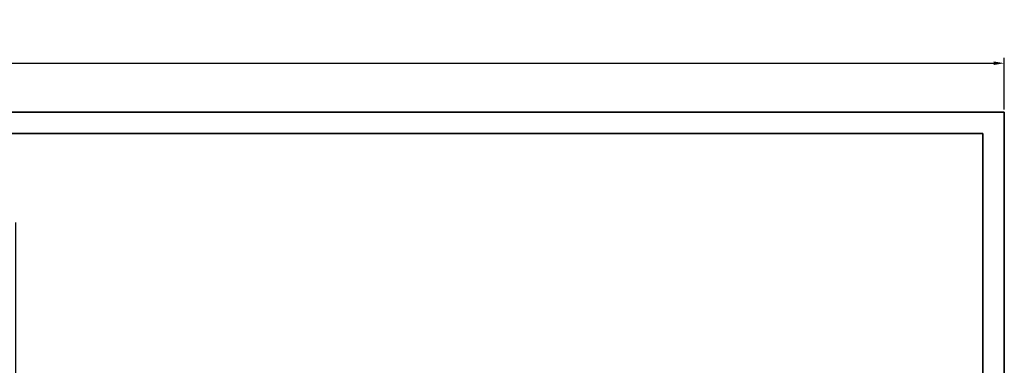
# Model space of a CAD drawing. Units: inches. Extents: x 3008 to 4088, y 1255 to 2137.
# Tile 30 of 30: x 3853 to 4083, y 1951 to 2031. Entities that reach past the tile are written whole.
import ezdxf

# ---------------------------------------------------------------- set-up
doc = ezdxf.new("R2010")
doc.units = ezdxf.units.IN
doc.layers.add('A-ANNO-DIMS', color=2, linetype='Continuous', lineweight=18)
doc.layers.add('C-PROP', color=1, linetype='Continuous', lineweight=35)
doc.styles.get("Standard").update_dxf_attribs({"font": 'arial.ttf'})
doc.dimstyles.new('ISO-25', dxfattribs={"dimtxt": 8, "dimasz": 2.5, "dimexe": 1.25, "dimexo": 0.625, "dimtad": 1, "dimdec": 1, "dimlunit": 3, "dimtxsty": 'Standard', "dimcen": 2.5, "dimadec": 0, "dimazin": 0, "dimtfac": 1, "dimtdec": 1, "dimtmove": 0, "dimatfit": 3, "dimfxl": 1, "dimarcsym": 0})

# ---------------------------------------------------------------- blocks, each defined once
blk = doc.blocks.new('*D31')
at = {"layer": 'A-ANNO-DIMS', "color": 0, "lineweight": -2, "transparency": 16777216}
for p, q in [((3602.94, 2010.35), (3602.94, 2022.41)), ((3605.44, 2021.16), (4080.44, 2021.16)), ((4082.94, 2010.35), (4082.94, 2022.41))]:
    blk.add_line(p, q, dxfattribs=at)
at = {"layer": 'A-ANNO-DIMS', "color": 0, "transparency": 16777216}
for points in [[(3605.44, 2021.58), (3605.44, 2020.74), (3602.94, 2021.16)], [(4080.44, 2021.58), (4080.44, 2020.74), (4082.94, 2021.16)]]:
    blk.add_solid(points, dxfattribs=at)
at = {"layer": 'Defpoints', "color": 0, "transparency": 16777216}
for p in [(4082.94, 2021.16), (3602.94, 2009.72), (4082.94, 2009.72)]:
    blk.add_point(p, dxfattribs=at)
at = {"layer": 'A-ANNO-DIMS', "color": 0, "transparency": 16777216, "insert": (3842.94, 2025.87), "char_height": 8, "attachment_point": 5}
blk.add_mtext("40'", dxfattribs=at)
blk = doc.blocks.new('*D47')
at = {"layer": 'A-ANNO-DIMS', "color": 0, "lineweight": -2, "transparency": 16777216}
for p, q in [((3852.13, 1857.83), (3852.13, 1983.94)), ((3853.47, 1857.83), (3850.88, 1857.83)), ((3852.13, 1847.22), (3852.13, 1855.33)), ((3853.47, 1844.72), (3850.88, 1844.72))]:
    blk.add_line(p, q, dxfattribs=at)
at = {"layer": 'A-ANNO-DIMS', "color": 0, "transparency": 16777216}
for points in [[(3851.71, 1855.33), (3852.54, 1855.33), (3852.13, 1857.83)], [(3851.71, 1847.22), (3852.54, 1847.22), (3852.13, 1844.72)]]:
    blk.add_solid(points, dxfattribs=at)
at = {"layer": 'Defpoints', "color": 0, "transparency": 16777216}
for p in [(3852.13, 1857.83), (3854.09, 1857.83), (3854.09, 1844.72)]:
    blk.add_point(p, dxfattribs=at)
at = {"layer": 'A-ANNO-DIMS', "color": 0, "transparency": 16777216, "insert": (3847.36, 1922.14), "char_height": 8, "attachment_point": 5, "rotation": 90}
blk.add_mtext('WASH BASIN 1\'-1" TYP.', dxfattribs=at)

msp = doc.modelspace()

# ---------------------------------------------------------------- linework, layer by layer
at = {"layer": 'C-PROP'}
for p, q in [((3602.94, 2009.72), (4082.94, 2009.72)), ((4082.94, 2009.72), (4082.94, 1349.72)), ((3607.94, 2004.72), (4077.94, 2004.72)), ((4077.94, 2004.72), (4077.94, 1354.72))]:
    msp.add_line(p, q, dxfattribs=at)

# ---------------------------------------------------------------- dimensions: what is measured, and where the dimension line sits
at = {"layer": 'A-ANNO-DIMS'}
dim = msp.add_linear_dim(base=(4082.94, 2021.16), p1=(3602.94, 2009.72), p2=(4082.94, 2009.72), dimstyle='ISO-25', override={"dimclrd": 0, "dimclre": 0, "dimclrt": 0}, dxfattribs=at)
dim.commit()
dim.dimension.update_dxf_attribs({"geometry": '*D31', "text_midpoint": (3842.94, 2025.87)})
dim = msp.add_linear_dim(base=(3852.13, 1857.83), p1=(3854.09, 1844.72), p2=(3854.09, 1857.83), angle=90, text='WASH BASIN <> TYP.', dimstyle='ISO-25', override={"dimdec": 1, "dimrnd": 0, "dimzin": 1, "dimlunit": 4, "dimfrac": 2}, dxfattribs=at)
dim.commit()
dim.dimension.update_dxf_attribs({"geometry": '*D47', "text_midpoint": (3847.36, 1922.14)})

doc.saveas('drawing.dxf')
